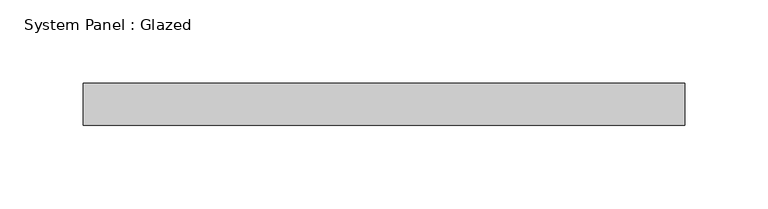
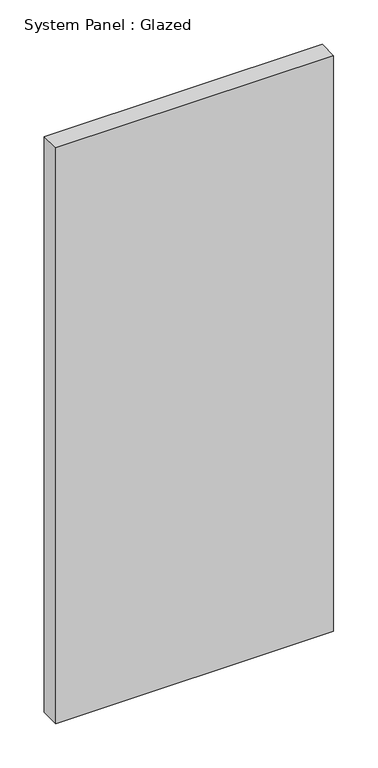
"""IFC4 building model written with IfcOpenShell, lengths in millimetres: plate geometry, System Panel : Glazed."""

from ifc_helpers import new_model, si_unit, origin, origin_with_axes, place, context, project, spatial, polyline, outline, extrude, source, transform, mapped, element, save


def system_panel_glazed_8fc33089(model_context):
    return source(origin(), model_context, "Body", "SweptSolid", [
        extrude(outline(polyline([(180.975, 19.05), (-180.975, 19.05), (-180.975, 44.45), (180.975, 44.45), (180.975, 19.05)])), origin_with_axes(), (0.0, 0.0, 1.0), 791.7415583),
    ])


if __name__ == "__main__":
    model = new_model("IFC4")
    model_context = context("Model", 3, world=origin())
    ifc_project = project(units=[si_unit("LENGTHUNIT", "METRE", prefix="MILLI")], contexts=[model_context])
    site = spatial("IfcSite", under=ifc_project)
    building = spatial("IfcBuilding", under=site)
    placement = place(None, origin())
    system_panel_glazed_shape = system_panel_glazed_8fc33089(model_context)
    element("IfcPlate", 1, ObjectType="System Panel : Glazed", at=placement, inside=building, context=model_context, shape_type="MappedRepresentation", body=[
        mapped(system_panel_glazed_shape, transform((0.0, 0.0, 0.0), x_axis=(1.0, 0.0, 0.0), y_axis=(0.0, 1.0, 0.0), z_axis=(0.0, 0.0, 1.0))),
    ])
    save(model, "model.ifc")

# Revit data of these elements
# Type "System Panel : Glazed"
#   Construction Type Id = "GSP4R"
#   Analytic Construction = "1/8 in Pilkington single glazing"
#   Visual Light Transmittance = 0.9
#   Solar Heat Gain Coefficient = 0.86
#   Heat Transfer Coefficient (U) = 1.18115 BTU/(h·ft²·°F)
#   Define Thermal Properties by = 1
# Element 1 (IfcPlate, "System Panel : Glazed")
#   Materials on its faces: "Glass"
# Materials
#   "Glass": class "Glass", colour RGB 0 128 192, transparency 0.75, Description = "Soda Lime Glass", Cost = 0
